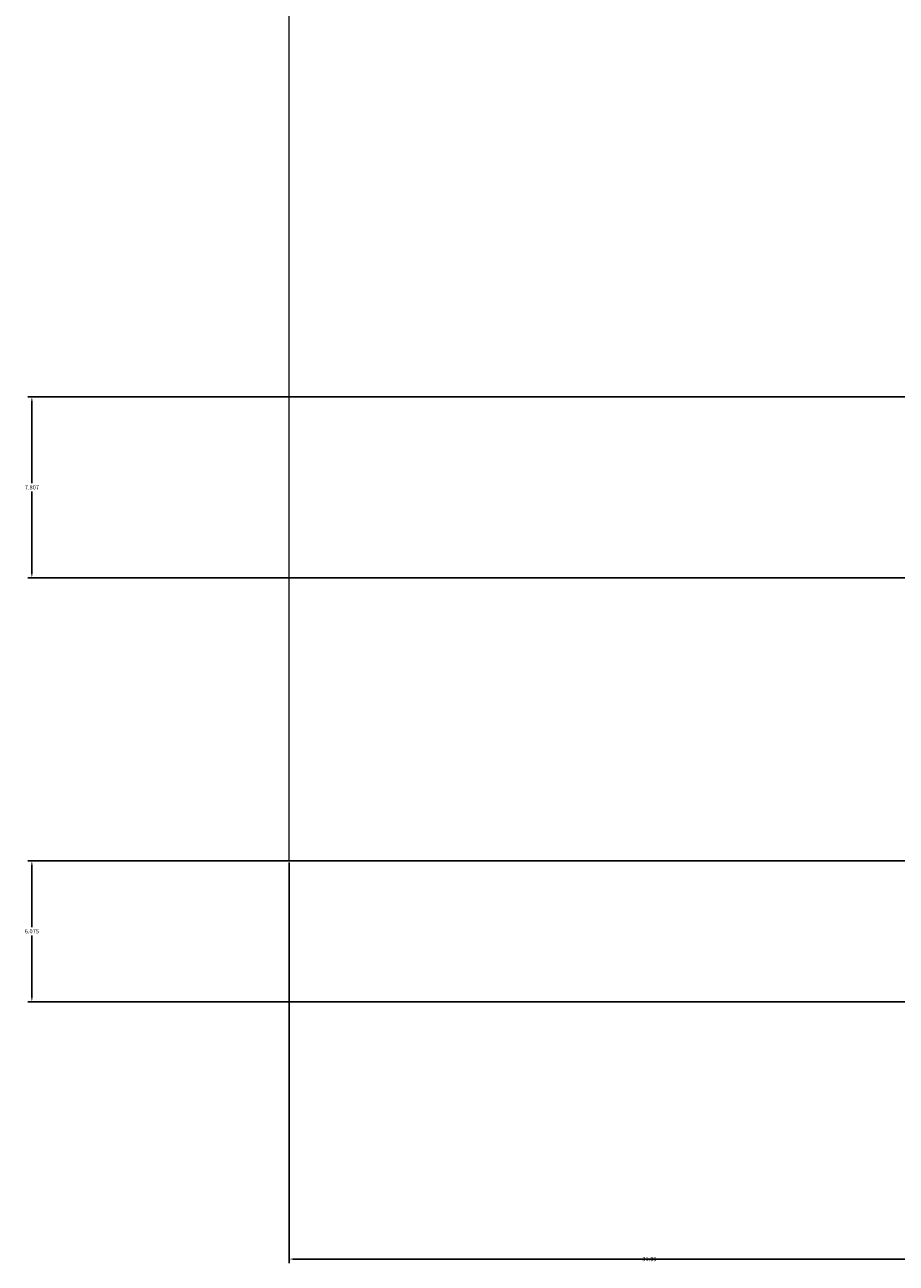
# Model space of a CAD drawing. Units: inches. Extents: x 412 to 584, y 208 to 437.
# Tile 1 of 28: x 412 to 450, y 208 to 262. Entities that reach past the tile are written whole.
import ezdxf

# ---------------------------------------------------------------- set-up
doc = ezdxf.new("R2010")
doc.units = ezdxf.units.IN
doc.header["$MEASUREMENT"] = 0
doc.layers.add('A-ANNO-DIMS', color=2, linetype='Continuous', lineweight=18)
doc.layers.add('E-ENCL', color=8, linetype='Continuous', lineweight=18)
doc.styles.get("Standard").update_dxf_attribs({"font": 'arial.ttf'})
doc.dimstyles.get("Standard").update_dxf_attribs({"dimtxt": 0.18, "dimasz": 0.18, "dimexe": 0.18, "dimexo": 0.0625, "dimgap": 0.09, "dimtad": 0, "dimtih": 1, "dimtoh": 1, "dimdec": 4, "dimzin": 0, "dimdsep": 46, "dimtxsty": 'Standard', "dimcen": 0.09, "dimadec": 0, "dimazin": 0, "dimtfac": 1, "dimtdec": 4, "dimtofl": 0, "dimtmove": 0, "dimatfit": 3, "dimfxl": 1, "dimtolj": 1, "dimtzin": 0, "dimarcsym": 0})

# ---------------------------------------------------------------- blocks, each defined once
blk = doc.blocks.new('*D13')
at = {"layer": 'A-ANNO-DIMS', "color": 0, "lineweight": -2, "transparency": 16777216}
for p, q in [((423.556, 225.526), (423.556, 208.233)), ((572.394, 225.526), (572.394, 208.233)), ((423.736, 208.413), (497.52, 208.413)), ((572.214, 208.413), (498.43, 208.413))]:
    blk.add_line(p, q, dxfattribs=at)
at = {"layer": 'A-ANNO-DIMS', "color": 0, "transparency": 16777216}
for points in [[(423.736, 208.443), (423.736, 208.383), (423.556, 208.413)], [(572.214, 208.443), (572.214, 208.383), (572.394, 208.413)]]:
    blk.add_solid(points, dxfattribs=at)
at = {"layer": 'Defpoints', "color": 0, "transparency": 16777216}
for p in [(423.556, 225.588), (572.394, 225.588), (572.394, 208.413)]:
    blk.add_point(p, dxfattribs=at)
at = {"layer": 'A-ANNO-DIMS', "color": 0, "transparency": 16777216, "insert": (497.975, 208.413), "char_height": 0.18, "attachment_point": 5}
blk.add_mtext('\\A1;148.84', dxfattribs=at)
blk = doc.blocks.new('*D14')
at = {"layer": 'A-ANNO-DIMS', "color": 0, "lineweight": -2, "transparency": 16777216}
for p, q in [((423.556, 225.526), (423.556, 208.233)), ((454.644, 219.451), (454.644, 208.233)), ((423.736, 208.413), (438.706, 208.413)), ((454.464, 208.413), (439.494, 208.413))]:
    blk.add_line(p, q, dxfattribs=at)
at = {"layer": 'A-ANNO-DIMS', "color": 0, "transparency": 16777216}
for points in [[(423.736, 208.443), (423.736, 208.383), (423.556, 208.413)], [(454.464, 208.443), (454.464, 208.383), (454.644, 208.413)]]:
    blk.add_solid(points, dxfattribs=at)
at = {"layer": 'Defpoints', "color": 0, "transparency": 16777216}
for p in [(423.556, 225.588), (454.644, 219.513), (454.644, 208.413)]:
    blk.add_point(p, dxfattribs=at)
at = {"layer": 'A-ANNO-DIMS', "color": 0, "transparency": 16777216, "insert": (439.1, 208.413), "char_height": 0.18, "attachment_point": 5}
blk.add_mtext('\\A1;31.09', dxfattribs=at)
blk = doc.blocks.new('*D37')
at = {"layer": 'A-ANNO-DIMS', "color": 0, "lineweight": -2, "transparency": 16777216}
for p, q in [((451.221, 245.604), (412.276, 245.604)), ((412.456, 245.424), (412.456, 241.882)), ((412.456, 237.977), (412.456, 241.518)), ((451.221, 237.797), (412.276, 237.797))]:
    blk.add_line(p, q, dxfattribs=at)
at = {"layer": 'A-ANNO-DIMS', "color": 0, "transparency": 16777216}
for points in [[(412.426, 245.424), (412.486, 245.424), (412.456, 245.604)], [(412.426, 237.977), (412.486, 237.977), (412.456, 237.797)]]:
    blk.add_solid(points, dxfattribs=at)
at = {"layer": 'Defpoints', "color": 0, "transparency": 16777216}
for p in [(451.283, 245.604), (412.456, 237.797), (451.283, 237.797)]:
    blk.add_point(p, dxfattribs=at)
at = {"layer": 'A-ANNO-DIMS', "color": 0, "transparency": 16777216, "insert": (412.456, 241.7), "char_height": 0.18, "attachment_point": 5}
blk.add_mtext('\\A1;7.807', dxfattribs=at)
blk = doc.blocks.new('*D38')
at = {"layer": 'A-ANNO-DIMS', "color": 0, "lineweight": -2, "transparency": 16777216}
for p, q in [((451.074, 225.588), (412.276, 225.588)), ((412.456, 225.408), (412.456, 222.733)), ((412.456, 219.693), (412.456, 222.369)), ((454.582, 219.513), (412.276, 219.513))]:
    blk.add_line(p, q, dxfattribs=at)
at = {"layer": 'A-ANNO-DIMS', "color": 0, "transparency": 16777216}
for points in [[(412.426, 225.408), (412.486, 225.408), (412.456, 225.588)], [(412.426, 219.693), (412.486, 219.693), (412.456, 219.513)]]:
    blk.add_solid(points, dxfattribs=at)
at = {"layer": 'Defpoints', "color": 0, "transparency": 16777216}
for p in [(451.137, 225.588), (412.456, 219.513), (454.644, 219.513)]:
    blk.add_point(p, dxfattribs=at)
at = {"layer": 'A-ANNO-DIMS', "color": 0, "transparency": 16777216, "insert": (412.456, 222.551), "char_height": 0.18, "attachment_point": 5}
blk.add_mtext('\\A1;6.075', dxfattribs=at)

msp = doc.modelspace()

# ---------------------------------------------------------------- linework, layer by layer
at = {"layer": 'E-ENCL'}
msp.add_lwpolyline([(423.5562, 309.3773), (572.3937, 309.3773), (572.3937, 225.5881), (423.5562, 225.5881)], close=True, dxfattribs=at)

# ---------------------------------------------------------------- dimensions: what is measured, and where the dimension line sits
at = {"layer": 'A-ANNO-DIMS'}
for base, p1, p2, picture, middle in [((412.4562, 237.797), (451.283, 245.6036), (451.283, 237.797), '*D37', (412.4562, 241.7003)), ((412.4562, 219.5133), (451.1367, 225.5881), (454.6441, 219.5133), '*D38', (412.4562, 222.5507))]:
    dim = msp.add_linear_dim(base=base, p1=p1, p2=p2, angle=90, dimstyle='Standard', override={"dimdec": 3, "dimlfac": 1, "dimrnd": 0, "dimzin": 0, "dimdsep": 46, "dimlunit": 2}, dxfattribs=at)
    dim.commit()
    dim.dimension.update_dxf_attribs({"geometry": picture, "text_midpoint": middle})
for base, p2, picture, middle in [((572.3937, 208.4133), (572.3937, 225.5881), '*D13', (497.975, 208.4133)), ((454.6441, 208.4133), (454.6441, 219.5133), '*D14', (439.1001, 208.4133))]:
    dim = msp.add_linear_dim(base=base, p1=(423.5562, 225.5881), p2=p2, dimstyle='Standard', override={"dimdec": 2, "dimlfac": 1, "dimrnd": 0, "dimzin": 0, "dimdsep": 46, "dimlunit": 2}, dxfattribs=at)
    dim.commit()
    dim.dimension.update_dxf_attribs({"geometry": picture, "text_midpoint": middle})

doc.saveas('drawing.dxf')
